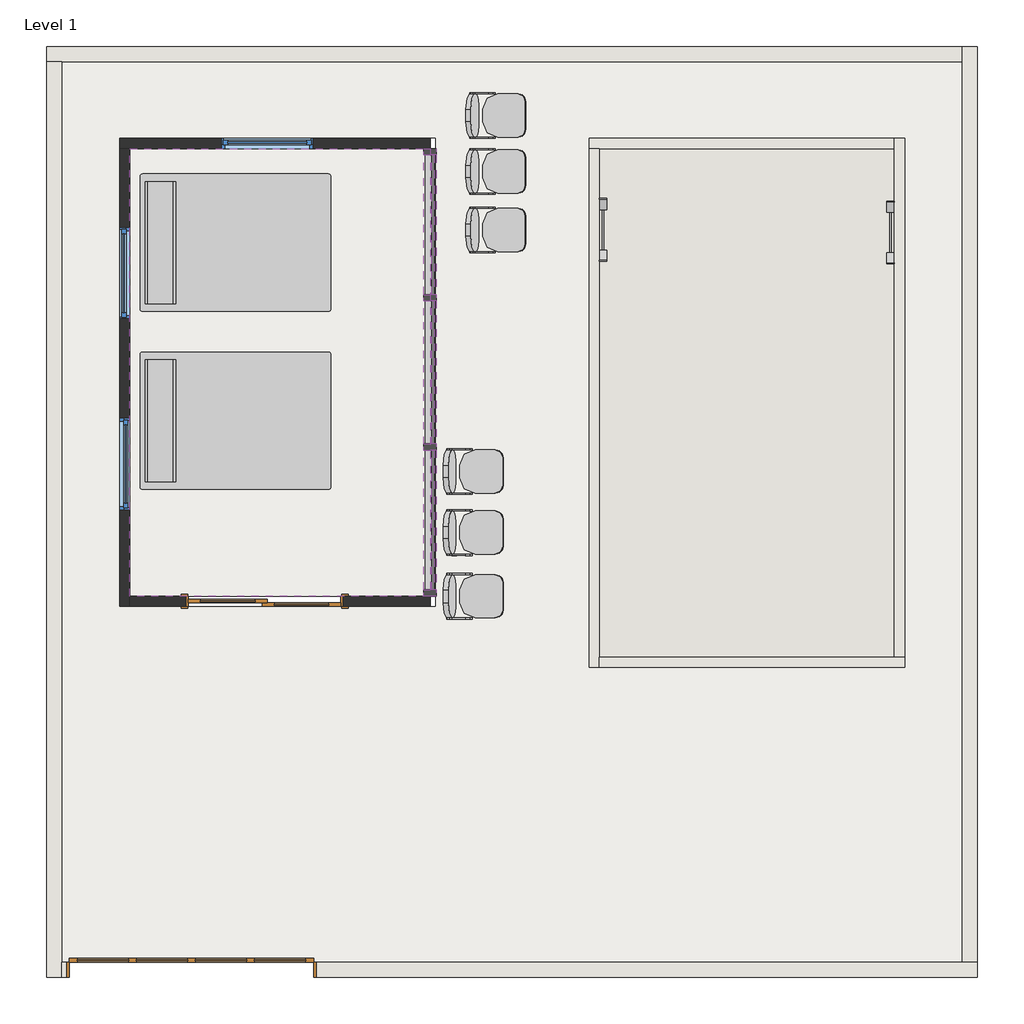
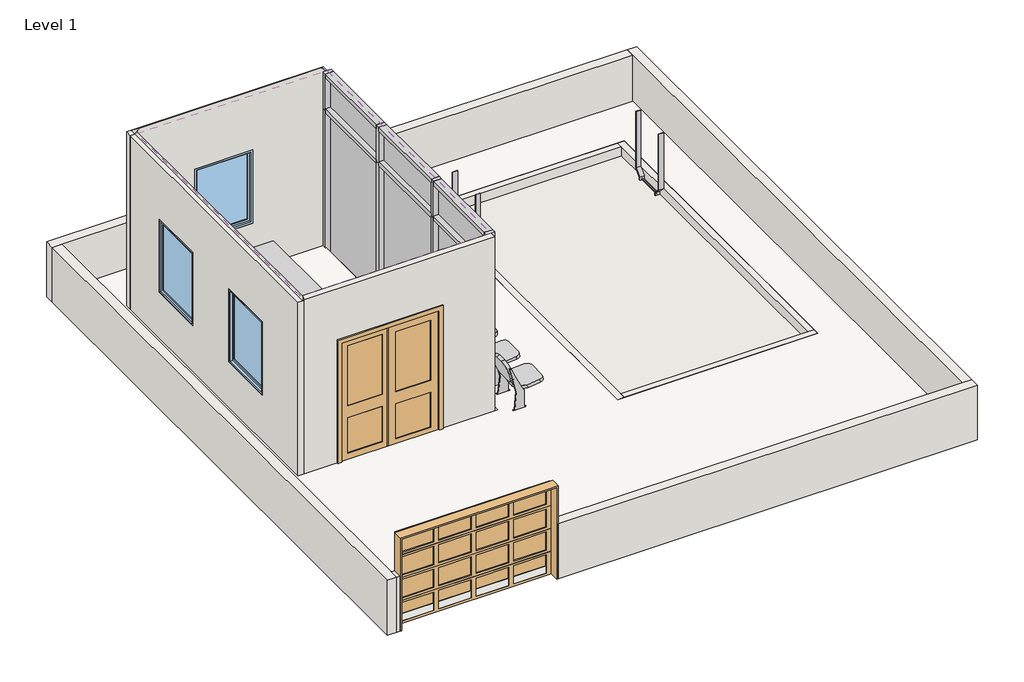
# One storey, incomplete: 17 members, 12 walls, 8 furniture elements, 6 plates, 3 slabs, 3 windows, 2 doors, 2 proxies, 1 covering.
"""IFC4 building model written with IfcOpenShell, lengths in millimetres."""

from ifc_helpers import new_model, si_unit, frame, origin, origin_with_axes, place, context, project, spatial, polyline, outline, extrude, faceted_brep, transform, mapped, element, save
from components import ladder_standard_19ab645e, ladder_standard_86d3c5fc, door_11e1ca51, m_door_interior_double_sliding_2_panel_wood_1524_x_2134mm_74d6d249, furniture_0253826f, m_seating_auditorium_457_x_610mm_3d1d9cbc, member_f0fea5a5, member_6e77e263, member_ee409385, member_47bfaf8a, member_2e151cea, member_16a3b7c2, member_950090be, member_3c30aa5e, system_panel_glazed_1fb160e7, system_panel_glazed_56a6bb10, system_panel_glazed_2f197d06, system_panel_glazed_b12e8a87, walls_1_walls_1_4e806b56, window_d45db805

model = new_model("IFC4")

# Units and contexts
model_context = context("Model", 3, world=origin())
ifc_project = project(units=[si_unit("LENGTHUNIT", "METRE", prefix="MILLI")], contexts=[model_context])

# Site, building, storey
site = spatial("IfcSite", under=ifc_project)
building = spatial("IfcBuilding", under=site)
storey = spatial("IfcBuildingStorey", under=building, Name="Level 1", Elevation=0.0)

# Proxies
placement = place(None, origin())
ladder_standard_shape = ladder_standard_19ab645e(model_context)
element("IfcBuildingElementProxy", 1, Name="Ladder : Standard", ObjectType="Ladder : Standard", at=placement, inside=storey, context=model_context, shape_type="MappedRepresentation", body=[
    mapped(ladder_standard_shape, transform((-3124.1401579, 11504.6599287, 19.05), x_axis=(0.0, 1.0, 0.0), y_axis=(-1.0, 0.0, 0.0), z_axis=(0.0, 0.0, 1.0))),
])
ladder_standard_2_shape = ladder_standard_86d3c5fc(model_context)
element("IfcBuildingElementProxy", 2, Name="Ladder : Standard", ObjectType="Ladder : Standard", at=placement, inside=storey, context=model_context, shape_type="MappedRepresentation", body=[
    mapped(ladder_standard_2_shape, transform((-6197.5401579, 11530.0599287, 0.0), x_axis=(0.0, -1.0, 0.0), y_axis=(1.0, 0.0, 0.0), z_axis=(0.0, 0.0, 1.0))),
])

# Covering
element("IfcCovering", 3, ObjectType="2' x 4' ACT System", at=placement, inside=storey, context=model_context, shape_type="SweptSolid", body=[
    extrude(outline(polyline([(-10822.8289971, 12342.8599287), (-7825.6289971, 12342.8599287), (-7825.6289971, 7872.4599287), (-10822.8289971, 7872.4599287), (-10822.8289971, 12342.8599287)])), frame((0.0, 0.0, 3048.0), z_axis=(0.0, 0.0, 1.0), x_axis=(1.0, 0.0, 0.0)), (0.0, 0.0, 1.0), 57.15),
])

# Doors
door_shape = door_11e1ca51(model_context)
element("IfcDoor", 4, ObjectType="Door-Garage-Embossed_Panel : 96\" x 60\"", at=placement, inside=storey, context=model_context, shape_type="MappedRepresentation", body=[
    mapped(door_shape, transform((-10207.2557492, 4138.1512164, 0.0), x_axis=(-1.0, 0.0, 0.0), y_axis=(0.0, -1.0, 0.0), z_axis=(0.0, 0.0, 1.0))),
])
m_door_interior_double_sliding_2_panel_wood_1524_x_2134mm_shape = m_door_interior_double_sliding_2_panel_wood_1524_x_2134mm_74d6d249(model_context)
element("IfcDoor", 5, ObjectType="M_Door-Interior-Double-Sliding-2_Panel-Wood : 1524 x 2134mm", at=placement, inside=storey, context=model_context, shape_type="MappedRepresentation", body=[
    mapped(m_door_interior_double_sliding_2_panel_wood_1524_x_2134mm_shape, transform((-9476.6289971, 7818.4849287, 0.0), x_axis=(-1.0, 0.0, 0.0), y_axis=(0.0, -1.0, 0.0), z_axis=(0.0, 0.0, 1.0))),
])

# Furniture
furniture_shape = furniture_0253826f(model_context)
element("IfcFurniture", 6, ObjectType="Bed-Standard : Double 54\" x 75\"", at=placement, inside=storey, context=model_context, shape_type="MappedRepresentation", body=[
    mapped(furniture_shape, transform((-9814.324079, 11131.5714041, 152.4), x_axis=(0.0, 1.0000000000000002, 0.0), y_axis=(-1.0000000000000002, 0.0, 0.0), z_axis=(0.0, 0.0, 1.0))),
])
element("IfcFurniture", 7, ObjectType="Bed-Standard : Double 54\" x 75\"", at=placement, inside=storey, context=model_context, shape_type="MappedRepresentation", body=[
    mapped(furniture_shape, transform((-9814.324079, 9353.5714041, 152.4), x_axis=(0.0, 1.0000000000000002, 0.0), y_axis=(-1.0000000000000002, 0.0, 0.0), z_axis=(0.0, 0.0, 1.0))),
])
m_seating_auditorium_457_x_610mm_shape = m_seating_auditorium_457_x_610mm_3d1d9cbc(model_context)
element("IfcFurniture", 8, ObjectType="M_Seating-Auditorium : 457 x 610mm", at=placement, inside=storey, context=model_context, shape_type="MappedRepresentation", body=[
    mapped(m_seating_auditorium_457_x_610mm_shape, transform((-7365.3155677, 12833.7877975, 152.4), x_axis=(0.0, -1.0, 0.0), y_axis=(1.0, 0.0, 0.0), z_axis=(0.0, 0.0, 1.0))),
])
element("IfcFurniture", 9, ObjectType="M_Seating-Auditorium : 457 x 610mm", at=placement, inside=storey, context=model_context, shape_type="MappedRepresentation", body=[
    mapped(m_seating_auditorium_457_x_610mm_shape, transform((-7365.3155677, 12274.9877975, 152.4), x_axis=(0.0, -1.0, 0.0), y_axis=(1.0, 0.0, 0.0), z_axis=(0.0, 0.0, 1.0))),
])
element("IfcFurniture", 10, ObjectType="M_Seating-Auditorium : 457 x 610mm", at=placement, inside=storey, context=model_context, shape_type="MappedRepresentation", body=[
    mapped(m_seating_auditorium_457_x_610mm_shape, transform((-7365.3155677, 11690.7877975, 152.4), x_axis=(0.0, -1.0, 0.0), y_axis=(1.0, 0.0, 0.0), z_axis=(0.0, 0.0, 1.0))),
])
element("IfcFurniture", 11, ObjectType="M_Seating-Auditorium : 457 x 610mm", at=placement, inside=storey, context=model_context, shape_type="MappedRepresentation", body=[
    mapped(m_seating_auditorium_457_x_610mm_shape, transform((-7593.9155677, 9277.7877975, 152.4), x_axis=(0.0, -1.0, 0.0), y_axis=(1.0, 0.0, 0.0), z_axis=(0.0, 0.0, 1.0))),
])
element("IfcFurniture", 12, ObjectType="M_Seating-Auditorium : 457 x 610mm", at=placement, inside=storey, context=model_context, shape_type="MappedRepresentation", body=[
    mapped(m_seating_auditorium_457_x_610mm_shape, transform((-7593.9155677, 8668.1877975, 152.4), x_axis=(0.0, -1.0, 0.0), y_axis=(1.0, 0.0, 0.0), z_axis=(0.0, 0.0, 1.0))),
])
element("IfcFurniture", 13, ObjectType="M_Seating-Auditorium : 457 x 610mm", at=placement, inside=storey, context=model_context, shape_type="MappedRepresentation", body=[
    mapped(m_seating_auditorium_457_x_610mm_shape, transform((-7593.9155677, 8033.1877975, 152.4), x_axis=(0.0, -1.0, 0.0), y_axis=(1.0, 0.0, 0.0), z_axis=(0.0, 0.0, 1.0))),
])

# Members
member_shape = member_f0fea5a5(model_context)
element("IfcMember", 14, ObjectType="Rectangular Mullion : 2.5\" x 5\" rectangular", at=placement, inside=storey, context=model_context, shape_type="MappedRepresentation", body=[
    mapped(member_shape, transform((-7825.6289971, 10852.7265953, 0.0), x_axis=(0.0, -1.0, 0.0), y_axis=(-1.0, 0.0, 0.0), z_axis=(0.0, 0.0, -1.0))),
])
element("IfcMember", 15, ObjectType="Rectangular Mullion : 2.5\" x 5\" rectangular", at=placement, inside=storey, context=model_context, shape_type="MappedRepresentation", body=[
    mapped(member_shape, transform((-7825.6289971, 9362.593262, 0.0), x_axis=(0.0, -1.0, 0.0), y_axis=(-1.0, 0.0, 0.0), z_axis=(0.0, 0.0, -1.0))),
])
member_2_shape = member_6e77e263(model_context)
element("IfcMember", 16, ObjectType="Rectangular Mullion : 2.5\" x 5\" rectangular", at=placement, inside=storey, context=model_context, shape_type="MappedRepresentation", body=[
    mapped(member_2_shape, transform((-7825.6289971, 10852.7265953, 2438.4), x_axis=(0.0, -1.0, 0.0), y_axis=(-1.0, 0.0, 0.0), z_axis=(0.0, 0.0, -1.0))),
])
element("IfcMember", 17, ObjectType="Rectangular Mullion : 2.5\" x 5\" rectangular", at=placement, inside=storey, context=model_context, shape_type="MappedRepresentation", body=[
    mapped(member_2_shape, transform((-7825.6289971, 9362.593262, 2438.4), x_axis=(0.0, -1.0, 0.0), y_axis=(-1.0, 0.0, 0.0), z_axis=(0.0, 0.0, -1.0))),
])
member_3_shape = member_ee409385(model_context)
element("IfcMember", 18, ObjectType="Rectangular Mullion : 2.5\" x 5\" rectangular", at=placement, inside=storey, context=model_context, shape_type="MappedRepresentation", body=[
    mapped(member_3_shape, transform((-7825.6289971, 7872.4599287, 0.0), x_axis=(0.0, -1.0, 0.0), y_axis=(-1.0, 0.0, 0.0), z_axis=(0.0, 0.0, -1.0))),
])
element("IfcMember", 19, ObjectType="Rectangular Mullion : 2.5\" x 5\" rectangular", at=placement, inside=storey, context=model_context, shape_type="MappedRepresentation", body=[
    mapped(member_3_shape, transform((-7825.6289971, 12342.8599287, 2438.4), x_axis=(0.0, 1.0, 0.0), y_axis=(-1.0, 0.0, 0.0), z_axis=(0.0, 0.0, 1.0))),
])
member_4_shape = member_47bfaf8a(model_context)
element("IfcMember", 20, ObjectType="Rectangular Mullion : 2.5\" x 5\" rectangular", at=placement, inside=storey, context=model_context, shape_type="MappedRepresentation", body=[
    mapped(member_4_shape, transform((-7825.6289971, 7872.4599287, 2438.4), x_axis=(0.0, -1.0, 0.0), y_axis=(-1.0, 0.0, 0.0), z_axis=(0.0, 0.0, -1.0))),
])
element("IfcMember", 21, ObjectType="Rectangular Mullion : 2.5\" x 5\" rectangular", at=placement, inside=storey, context=model_context, shape_type="MappedRepresentation", body=[
    mapped(member_4_shape, transform((-7825.6289971, 12342.8599287, 3048.0), x_axis=(0.0, 1.0, 0.0), y_axis=(-1.0, 0.0, 0.0), z_axis=(0.0, 0.0, 1.0))),
])
member_5_shape = member_2e151cea(model_context)
element("IfcMember", 22, ObjectType="Rectangular Mullion : 2.5\" x 5\" rectangular", at=placement, inside=storey, context=model_context, shape_type="MappedRepresentation", body=[
    mapped(member_5_shape, transform((-7825.6289971, 10820.9765953, 0.0), x_axis=(0.0, 0.0, -1.0), y_axis=(-1.0, 0.0, 0.0), z_axis=(0.0, 1.0, 0.0))),
])
member_6_shape = member_16a3b7c2(model_context)
element("IfcMember", 23, ObjectType="Rectangular Mullion : 2.5\" x 5\" rectangular", at=placement, inside=storey, context=model_context, shape_type="MappedRepresentation", body=[
    mapped(member_6_shape, transform((-7825.6289971, 12279.3599287, 0.0), x_axis=(0.0, 0.0, -1.0), y_axis=(-1.0, 0.0, 0.0), z_axis=(0.0, 1.0, 0.0))),
])
element("IfcMember", 24, ObjectType="Rectangular Mullion : 2.5\" x 5\" rectangular", at=placement, inside=storey, context=model_context, shape_type="MappedRepresentation", body=[
    mapped(member_6_shape, transform((-7825.6289971, 9330.843262, 0.0), x_axis=(0.0, 0.0, -1.0), y_axis=(-1.0, 0.0, 0.0), z_axis=(0.0, 1.0, 0.0))),
])
element("IfcMember", 25, ObjectType="Rectangular Mullion : 2.5\" x 5\" rectangular", at=placement, inside=storey, context=model_context, shape_type="MappedRepresentation", body=[
    mapped(member_6_shape, transform((-7825.6289971, 7935.9599287, 3048.0), x_axis=(0.0, 0.0, 1.0), y_axis=(-1.0, 0.0, 0.0), z_axis=(0.0, -1.0, 0.0))),
])
element("IfcMember", 26, ObjectType="Rectangular Mullion : 2.5\" x 5\" rectangular", at=placement, inside=storey, context=model_context, shape_type="MappedRepresentation", body=[
    mapped(member_6_shape, transform((-7825.6289971, 10884.4765953, 3048.0), x_axis=(0.0, 0.0, 1.0), y_axis=(-1.0, 0.0, 0.0), z_axis=(0.0, -1.0, 0.0))),
])
element("IfcMember", 27, ObjectType="Rectangular Mullion : 2.5\" x 5\" rectangular", at=placement, inside=storey, context=model_context, shape_type="MappedRepresentation", body=[
    mapped(member_5_shape, transform((-7825.6289971, 9394.343262, 3048.0), x_axis=(0.0, 0.0, 1.0), y_axis=(-1.0, 0.0, 0.0), z_axis=(0.0, -1.0, 0.0))),
])
member_7_shape = member_950090be(model_context)
element("IfcMember", 28, ObjectType="Rectangular Mullion : 2.5\" x 5\" rectangular", at=placement, inside=storey, context=model_context, shape_type="MappedRepresentation", body=[
    mapped(member_7_shape, transform((-7825.6289971, 10884.4765953, 2438.4), x_axis=(0.0, 0.0, 1.0), y_axis=(-1.0, 0.0, 0.0), z_axis=(0.0, -1.0, 0.0))),
])
element("IfcMember", 29, ObjectType="Rectangular Mullion : 2.5\" x 5\" rectangular", at=placement, inside=storey, context=model_context, shape_type="MappedRepresentation", body=[
    mapped(member_7_shape, transform((-7825.6289971, 7935.9599287, 2438.4), x_axis=(0.0, 0.0, 1.0), y_axis=(-1.0, 0.0, 0.0), z_axis=(0.0, -1.0, 0.0))),
])
member_8_shape = member_3c30aa5e(model_context)
element("IfcMember", 30, ObjectType="Rectangular Mullion : 2.5\" x 5\" rectangular", at=placement, inside=storey, context=model_context, shape_type="MappedRepresentation", body=[
    mapped(member_8_shape, transform((-7825.6289971, 9394.343262, 2438.4), x_axis=(0.0, 0.0, 1.0), y_axis=(-1.0, 0.0, 0.0), z_axis=(0.0, -1.0, 0.0))),
])

# Plates
system_panel_glazed_shape = system_panel_glazed_1fb160e7(model_context)
element("IfcPlate", 31, ObjectType="System Panel : Glazed", at=placement, inside=storey, context=model_context, shape_type="MappedRepresentation", body=[
    mapped(system_panel_glazed_shape, transform((-7825.6289971, 11581.918262, 63.5), x_axis=(0.0, -1.0, 0.0), y_axis=(1.0, 0.0, 0.0), z_axis=(0.0, 0.0, 1.0))),
])
element("IfcPlate", 32, ObjectType="System Panel : Glazed", at=placement, inside=storey, context=model_context, shape_type="MappedRepresentation", body=[
    mapped(system_panel_glazed_shape, transform((-7825.6289971, 8633.4015953, 63.5), x_axis=(0.0, -1.0, 0.0), y_axis=(1.0, 0.0, 0.0), z_axis=(0.0, 0.0, 1.0))),
])
system_panel_glazed_2_shape = system_panel_glazed_56a6bb10(model_context)
element("IfcPlate", 33, ObjectType="System Panel : Glazed", at=placement, inside=storey, context=model_context, shape_type="MappedRepresentation", body=[
    mapped(system_panel_glazed_2_shape, transform((-7825.6289971, 10107.6599287, 63.5), x_axis=(0.0, -1.0, 0.0), y_axis=(1.0, 0.0, 0.0), z_axis=(0.0, 0.0, 1.0))),
])
system_panel_glazed_3_shape = system_panel_glazed_2f197d06(model_context)
element("IfcPlate", 34, ObjectType="System Panel : Glazed", at=placement, inside=storey, context=model_context, shape_type="MappedRepresentation", body=[
    mapped(system_panel_glazed_3_shape, transform((-7825.6289971, 11581.918262, 2470.15), x_axis=(0.0, -1.0, 0.0), y_axis=(1.0, 0.0, 0.0), z_axis=(0.0, 0.0, 1.0))),
])
element("IfcPlate", 35, ObjectType="System Panel : Glazed", at=placement, inside=storey, context=model_context, shape_type="MappedRepresentation", body=[
    mapped(system_panel_glazed_3_shape, transform((-7825.6289971, 8633.4015953, 2470.15), x_axis=(0.0, -1.0, 0.0), y_axis=(1.0, 0.0, 0.0), z_axis=(0.0, 0.0, 1.0))),
])
system_panel_glazed_4_shape = system_panel_glazed_b12e8a87(model_context)
element("IfcPlate", 36, ObjectType="System Panel : Glazed", at=placement, inside=storey, context=model_context, shape_type="MappedRepresentation", body=[
    mapped(system_panel_glazed_4_shape, transform((-7825.6289971, 10107.6599287, 2470.15), x_axis=(0.0, -1.0, 0.0), y_axis=(1.0, 0.0, 0.0), z_axis=(0.0, 0.0, 1.0))),
])

# Slabs
element("IfcSlab", 37, ObjectType="3\"", at=placement, inside=storey, context=model_context, shape_type="SweptSolid", body=[
    extrude(outline(polyline([(-3187.6401579, 12342.8599287), (-3187.6401579, 7262.8599287), (-6134.0401579, 7262.8599287), (-6134.0401579, 12342.8599287), (-3187.6401579, 12342.8599287)])), frame((0.0, 0.0, -1905.0), z_axis=(0.0, 0.0, 1.0), x_axis=(1.0, 0.0, 0.0)), (0.0, 0.0, 1.0), 76.2),
])
element("IfcSlab", 38, ObjectType="4\"", at=placement, inside=storey, context=model_context, shape_type="SweptSolid", body=[
    extrude(outline(polyline([(-7876.4289971, 12342.8599287), (-7876.4289971, 7872.4599287), (-10822.8289971, 7872.4599287), (-10822.8289971, 12342.8599287), (-7876.4289971, 12342.8599287)])), frame((0.0, 0.0, 50.8), z_axis=(0.0, 0.0, 1.0), x_axis=(1.0, 0.0, 0.0)), (0.0, 0.0, 1.0), 101.6),
])
element("IfcSlab", 39, ObjectType="6\"", at=placement, inside=storey, context=model_context, shape_type="SweptSolid", body=[
    extrude(outline(polyline([(-11502.6557492, 13209.1262164), (-2511.0557492, 13209.1262164), (-2511.0557492, 4217.5262164), (-11502.6557492, 4217.5262164), (-11502.6557492, 13209.1262164)]), holes=[polyline([(-3086.0401579, 7161.2599287), (-3086.0401579, 12444.4599287), (-6235.6401579, 12444.4599287), (-6235.6401579, 7161.2599287), (-3086.0401579, 7161.2599287)]), polyline([(-7774.8289971, 12444.4599287), (-10924.4289971, 12444.4599287), (-10924.4289971, 7770.8599287), (-7774.8289971, 7770.8599287), (-7774.8289971, 12444.4599287)])]), origin_with_axes(), (0.0, 0.0, 1.0), 152.4),
])

# Walls
element("IfcWall", 40, ObjectType="4\"", at=placement, inside=storey, context=model_context, shape_type="Brep", body=[
    faceted_brep([(-10924.4289971, 12342.8599287, 0.0), (-10822.8289971, 12342.8599287, 0.0), (-7825.6289971, 12342.8599287, 0.0), (-7825.6289971, 12342.8599287, 3048.0), (-7848.8563022, 12342.8599287, 3048.0), (-7914.5243913, 12342.8599287, 3124.2), (-10784.7336028, 12342.8599287, 3124.2), (-10822.8289971, 12342.8599287, 3079.99483), (-10850.401692, 12342.8599287, 3048.0), (-10924.4289971, 12342.8599287, 3048.0), (-8994.0289971, 12342.8599287, 2133.6), (-8994.0289971, 12342.8599287, 914.4), (-9908.4289971, 12342.8599287, 914.4), (-9908.4289971, 12342.8599287, 2133.6), (-10924.4289971, 12444.4599287, 0.0), (-10924.4289971, 12444.4599287, 3048.0), (-10850.401692, 12444.4599287, 3048.0), (-7848.8563022, 12444.4599287, 3048.0), (-7825.6289971, 12444.4599287, 3048.0), (-7825.6289971, 12444.4599287, 0.0), (-8994.0289971, 12444.4599287, 2133.6), (-9908.4289971, 12444.4599287, 2133.6), (-9908.4289971, 12444.4599287, 914.4), (-8994.0289971, 12444.4599287, 914.4)], [[[0, 1, 2, 3, 4, 5, 6, 7, 8, 9], [10, 11, 12, 13]], [[14, 15, 16, 17, 18, 19], [20, 21, 22, 23]], [[2, 1, 0, 14, 19]], [[3, 2, 19, 18]], [[0, 9, 15, 14]], [[9, 8, 16, 15]], [[8, 7, 6, 16]], [[6, 5, 17, 16]], [[5, 4, 17]], [[4, 3, 18, 17]], [[11, 10, 20, 23]], [[12, 11, 23, 22]], [[13, 12, 22, 21]], [[10, 13, 21, 20]]]),
])
element("IfcWall", 41, ObjectType="4\"", at=placement, inside=storey, context=model_context, shape_type="Brep", body=[
    faceted_brep([(-10822.8289971, 7770.8599287, 0.0), (-10822.8289971, 7872.4599287, 0.0), (-10822.8289971, 12342.8599287, 0.0), (-10822.8289971, 12342.8599287, 3079.99483), (-10822.8289971, 7813.5197021, 3079.99483), (-10822.8289971, 7770.8599287, 3048.0), (-10822.8289971, 8736.0599287, 2133.6), (-10822.8289971, 9650.4599287, 2133.6), (-10822.8289971, 9650.4599287, 914.4), (-10822.8289971, 8736.0599287, 914.4), (-10822.8289971, 11555.4599287, 2133.6), (-10822.8289971, 11555.4599287, 914.4), (-10822.8289971, 10641.0599287, 914.4), (-10822.8289971, 10641.0599287, 2133.6), (-10924.4289971, 7770.8599287, 0.0), (-10924.4289971, 7770.8599287, 3048.0), (-10924.4289971, 12342.8599287, 3048.0), (-10924.4289971, 12342.8599287, 0.0), (-10924.4289971, 8736.0599287, 2133.6), (-10924.4289971, 8736.0599287, 914.4), (-10924.4289971, 9650.4599287, 914.4), (-10924.4289971, 9650.4599287, 2133.6), (-10924.4289971, 11555.4599287, 2133.6), (-10924.4289971, 10641.0599287, 2133.6), (-10924.4289971, 10641.0599287, 914.4), (-10924.4289971, 11555.4599287, 914.4), (-10850.401692, 12342.8599287, 3048.0), (-10850.401692, 7770.8599287, 3048.0)], [[[0, 1, 2, 3, 4, 5], [6, 7, 8, 9], [10, 11, 12, 13]], [[14, 15, 16, 17], [18, 19, 20, 21], [22, 23, 24, 25]], [[2, 1, 0, 14, 17]], [[3, 2, 17, 16, 26]], [[5, 4, 27]], [[4, 3, 26, 27]], [[26, 16, 15, 27]], [[0, 5, 27, 15, 14]], [[19, 18, 6, 9]], [[20, 19, 9, 8]], [[21, 20, 8, 7]], [[18, 21, 7, 6]], [[11, 10, 22, 25]], [[12, 11, 25, 24]], [[13, 12, 24, 23]], [[10, 13, 23, 22]]]),
])
element("IfcWall", 42, ObjectType="4\"", at=placement, inside=storey, context=model_context, shape_type="SweptSolid", body=[
    extrude(outline(polyline([(0.0, -7825.6289971), (3048.0, -7825.6289971), (3048.0, -10822.8289971), (0.0, -10822.8289971), (0.0, -10263.6289971), (2158.6, -10263.6289971), (2158.6, -8689.6289971), (0.0, -8689.6289971), (0.0, -7825.6289971)])), frame((0.0, 7770.8599287, 0.0), z_axis=(0.0, 1.0, 0.0), x_axis=(0.0, 0.0, 1.0)), (0.0, 0.0, 1.0), 101.6),
])
element("IfcWall", 43, ObjectType="4\" 2", at=placement, inside=storey, context=model_context, shape_type="Brep", body=[
    faceted_brep([(-6235.6401579, 12342.8599287, -1828.8), (-6134.0401579, 12342.8599287, -1828.8), (-3187.6401579, 12342.8599287, -1828.8), (-3187.6401579, 12342.8599287, 152.4), (-6134.0401579, 12342.8599287, 152.4), (-6235.6401579, 12342.8599287, 152.4), (-6235.6401579, 12444.4599287, -1828.8), (-6235.6401579, 12444.4599287, 152.4), (-3187.6401579, 12444.4599287, 152.4), (-3187.6401579, 12444.4599287, -1828.8)], [[[0, 1, 2, 3, 4, 5]], [[6, 7, 8, 9]], [[2, 1, 0, 6, 9]], [[5, 4, 3, 8, 7]], [[0, 5, 7, 6]], [[3, 2, 9, 8]]]),
])
element("IfcWall", 44, ObjectType="4\" 2", at=placement, inside=storey, context=model_context, shape_type="Brep", body=[
    faceted_brep([(-6134.0401579, 7161.2599287, -1828.8), (-6134.0401579, 7262.8599287, -1828.8), (-6134.0401579, 12342.8599287, -1828.8), (-6134.0401579, 12342.8599287, 152.4), (-6134.0401579, 7262.8599287, 152.4), (-6134.0401579, 7161.2599287, 152.4), (-6235.6401579, 7161.2599287, -1828.8), (-6235.6401579, 7161.2599287, 152.4), (-6235.6401579, 12342.8599287, 152.4), (-6235.6401579, 12342.8599287, -1828.8)], [[[0, 1, 2, 3, 4, 5]], [[6, 7, 8, 9]], [[2, 1, 0, 6, 9]], [[5, 4, 3, 8, 7]], [[0, 5, 7, 6]], [[3, 2, 9, 8]]]),
])
element("IfcWall", 45, ObjectType="4\" 2", at=placement, inside=storey, context=model_context, shape_type="Brep", body=[
    faceted_brep([(-3086.0401579, 7262.8599287, -1828.8), (-3187.6401579, 7262.8599287, -1828.8), (-6134.0401579, 7262.8599287, -1828.8), (-6134.0401579, 7262.8599287, 152.4), (-3187.6401579, 7262.8599287, 152.4), (-3086.0401579, 7262.8599287, 152.4), (-3086.0401579, 7161.2599287, -1828.8), (-3086.0401579, 7161.2599287, 152.4), (-6134.0401579, 7161.2599287, 152.4), (-6134.0401579, 7161.2599287, -1828.8)], [[[0, 1, 2, 3, 4, 5]], [[6, 7, 8, 9]], [[2, 1, 0, 6, 9]], [[5, 4, 3, 8, 7]], [[0, 5, 7, 6]], [[3, 2, 9, 8]]]),
])
element("IfcWall", 46, ObjectType="4\" 2", at=placement, inside=storey, context=model_context, shape_type="Brep", body=[
    faceted_brep([(-3187.6401579, 12444.4599287, -1828.8), (-3187.6401579, 12342.8599287, -1828.8), (-3187.6401579, 7262.8599287, -1828.8), (-3187.6401579, 7262.8599287, 152.4), (-3187.6401579, 12342.8599287, 152.4), (-3187.6401579, 12444.4599287, 152.4), (-3086.0401579, 12444.4599287, -1828.8), (-3086.0401579, 12444.4599287, 152.4), (-3086.0401579, 7262.8599287, 152.4), (-3086.0401579, 7262.8599287, -1828.8)], [[[0, 1, 2, 3, 4, 5]], [[6, 7, 8, 9]], [[2, 1, 0, 6, 9]], [[5, 4, 3, 8, 7]], [[0, 5, 7, 6]], [[3, 2, 9, 8]]]),
])
element("IfcWall", 47, ObjectType="6\"", at=placement, inside=storey, context=model_context, shape_type="Brep", body=[
    faceted_brep([(-11655.0557492, 13209.1262164, 0.0), (-11502.6557492, 13209.1262164, 0.0), (-2511.0557492, 13209.1262164, 0.0), (-2511.0557492, 13209.1262164, 914.4), (-11502.6557492, 13209.1262164, 914.4), (-11655.0557492, 13209.1262164, 914.4), (-11655.0557492, 13361.5262164, 0.0), (-11655.0557492, 13361.5262164, 914.4), (-2511.0557492, 13361.5262164, 914.4), (-2511.0557492, 13361.5262164, 0.0)], [[[0, 1, 2, 3, 4, 5]], [[6, 7, 8, 9]], [[2, 1, 0, 6, 9]], [[5, 4, 3, 8, 7]], [[0, 5, 7, 6]], [[3, 2, 9, 8]]]),
])
element("IfcWall", 48, ObjectType="6\"", at=placement, inside=storey, context=model_context, shape_type="Brep", body=[
    faceted_brep([(-11502.6557492, 4065.1262164, 0.0), (-11502.6557492, 4217.5262164, 0.0), (-11502.6557492, 13209.1262164, 0.0), (-11502.6557492, 13209.1262164, 914.4), (-11502.6557492, 4217.5262164, 914.4), (-11502.6557492, 4065.1262164, 914.4), (-11655.0557492, 4065.1262164, 0.0), (-11655.0557492, 4065.1262164, 914.4), (-11655.0557492, 13209.1262164, 914.4), (-11655.0557492, 13209.1262164, 0.0)], [[[0, 1, 2, 3, 4, 5]], [[6, 7, 8, 9]], [[2, 1, 0, 6, 9]], [[5, 4, 3, 8, 7]], [[0, 5, 7, 6]], [[3, 2, 9, 8]]]),
])
element("IfcWall", 49, ObjectType="6\"", at=placement, inside=storey, context=model_context, shape_type="Brep", body=[
    faceted_brep([(-11502.6557492, 4217.5262164, 0.0), (-11502.6557492, 4217.5262164, 914.4), (-11451.8557492, 4217.5262164, 914.4), (-11451.8557492, 4217.5262164, 0.0), (-11502.6557492, 4065.1262164, 914.4), (-11502.6557492, 4065.1262164, 0.0), (-11451.8557492, 4065.1262164, 0.0), (-11451.8557492, 4065.1262164, 914.4)], [[[0, 1, 2, 3]], [[4, 5, 6, 7]], [[5, 0, 3, 6]], [[1, 4, 7, 2]], [[1, 0, 5, 4]], [[3, 2, 7, 6]]]),
    faceted_brep([(-2358.6557492, 4217.5262164, 914.4), (-2358.6557492, 4217.5262164, 0.0), (-2511.0557492, 4217.5262164, 0.0), (-8962.6557492, 4217.5262164, 0.0), (-8962.6557492, 4217.5262164, 914.4), (-2511.0557492, 4217.5262164, 914.4), (-2358.6557492, 4065.1262164, 0.0), (-2358.6557492, 4065.1262164, 914.4), (-8962.6557492, 4065.1262164, 914.4), (-8962.6557492, 4065.1262164, 0.0)], [[[0, 1, 2, 3, 4, 5]], [[6, 7, 8, 9]], [[1, 6, 9, 3, 2]], [[7, 0, 5, 4, 8]], [[1, 0, 7, 6]], [[4, 3, 9, 8]]]),
])
element("IfcWall", 50, ObjectType="6\"", at=placement, inside=storey, context=model_context, shape_type="Brep", body=[
    faceted_brep([(-2511.0557492, 13361.5262164, 0.0), (-2511.0557492, 13209.1262164, 0.0), (-2511.0557492, 4217.5262164, 0.0), (-2511.0557492, 4217.5262164, 914.4), (-2511.0557492, 13209.1262164, 914.4), (-2511.0557492, 13361.5262164, 914.4), (-2358.6557492, 13361.5262164, 0.0), (-2358.6557492, 13361.5262164, 914.4), (-2358.6557492, 4217.5262164, 914.4), (-2358.6557492, 4217.5262164, 0.0)], [[[0, 1, 2, 3, 4, 5]], [[6, 7, 8, 9]], [[2, 1, 0, 6, 9]], [[5, 4, 3, 8, 7]], [[0, 5, 7, 6]], [[3, 2, 9, 8]]]),
])
walls_1_walls_1_shape = walls_1_walls_1_4e806b56(model_context)
element("IfcWall", 51, ObjectType="Walls 1 : Walls 1", at=placement, inside=storey, context=model_context, shape_type="MappedRepresentation", body=[
    mapped(walls_1_walls_1_shape, transform((0.0, 0.0, 0.0), x_axis=(1.0, 0.0, 0.0), y_axis=(0.0, 1.0, 0.0), z_axis=(0.0, 0.0, 1.0))),
])

# Windows
window_shape = window_d45db805(model_context)
element("IfcWindow", 52, ObjectType="Fixed : 36\" x 48\"", at=placement, inside=storey, context=model_context, shape_type="MappedRepresentation", body=[
    mapped(window_shape, transform((-10873.6289971, 9155.1599287, 0.0), x_axis=(0.0, -1.0, 0.0), y_axis=(1.0, 0.0, 0.0), z_axis=(0.0, 0.0, 1.0))),
])
element("IfcWindow", 53, ObjectType="Fixed : 36\" x 48\"", at=placement, inside=storey, context=model_context, shape_type="MappedRepresentation", body=[
    mapped(window_shape, transform((-10873.6289971, 11136.3599287, 0.0), x_axis=(0.0, 1.0, 0.0), y_axis=(-1.0, 0.0, 0.0), z_axis=(0.0, 0.0, 1.0))),
])
element("IfcWindow", 54, ObjectType="Fixed : 36\" x 48\"", at=placement, inside=storey, context=model_context, shape_type="MappedRepresentation", body=[
    mapped(window_shape, transform((-9413.1289971, 12393.6599287, 0.0), x_axis=(1.0, 0.0, 0.0), y_axis=(0.0, 1.0, 0.0), z_axis=(0.0, 0.0, 1.0))),
])

save(model, "model.ifc")

# Revit data of these elements
# Type "Ladder : Standard"
#   Rung Radius = 0' - 0 3/8"
#   Rung Length [instance default] = 1' - 4"
#   Side Rail Thickness = 0' - 3"
#   Side Rail Width = 0' - 0 3/8"
#   Half Guardrail Height = 1' - 9"
#   Height [instance default] = 15' - 2 1/2"
#   Guardrail Length = 1' - 8"
#   Guardrail Height = 3' - 6"
#   Distance [instance default] = 0' - 7"
#   Rung Space [instance default] = 1' - 0"
#   Number of Rungs [instance default] = 15
#   Default Elevation = 0
# Type "2' x 4' ACT System"
#   Assembly Code = "C3030210"
#   built-in parameter 1002203 = 1 (stored number, unit not read)
#   built-in parameter 1002202 = 1 (stored number, unit not read)
#   Layers, outside or top first: 0' - 1 5/8" "Default" (function 1); 0' - 0 5/8" "INT WALL" (function 5)
# Type "Door-Garage-Embossed_Panel : 96\" x 60\""
#   Type Mark = "10"
#   Assembly Code = "B2030400"
#   Analytic Construction = "Metal"
#   Thickness = 0' - 1 1/2"
#   Thermal Resistance (R) = 1.5338 (h·ft²·°F)/BTU
#   Rough Width = 8' - 2"
#   Rough Height = 5' - 1"
#   Panel Height = 1' - 3"
#   Height = 5' - 0"
#   Width = 8' - 0"
#   Heat Transfer Coefficient (U) = 0.6520 BTU/(h·ft²·°F)
#   Panels = 4
#   Function = 1
#   Exterior Trim [instance default] = yes
#   Trim Material = Steel, Paint Finish, Ivory, Matte
#   Panel Material = Steel, Paint Finish, Ivory, Matte
#   Frame Material = Steel, Paint Finish, Ivory, Matte
#   Visual Light Transmittance = 0
#   Solar Heat Gain Coefficient = 0
#   Wall Closure = (empty or 0)
# Type "M_Door-Interior-Double-Sliding-2_Panel-Wood : 1524 x 2134mm"
#   Type Mark = "9"
#   Assembly Code = "C1020300"
#   Analytic Construction = "Wooden"
#   Top Rail = 0' - 4.72441"
#   Thickness = 0' - 1.37795"
#   Thermal Resistance (R) = 2.5876 (h·ft²·°F)/BTU
#   Stiles = 0' - 4.72441"
#   Rough Width = 5' - 1.9685"
#   Rough Height = 7' - 0.98425"
#   Lock Rail = 0' - 7.87402"
#   Height = 7' - 0"
#   Width = 5' - 0"
#   Heat Transfer Coefficient (U) = 0.3865 BTU/(h·ft²·°F)
#   Bottom Rail = 0' - 9.05512"
#   Trim Material = Cherry
#   Panel Material = Cherry
#   Frame Material = Cherry
#   Visual Light Transmittance = 0
#   Solar Heat Gain Coefficient = 0
#   Wall Closure = (empty or 0)
#   Function = (empty or 0)
# Type "Bed-Standard : Double 54\" x 75\""
#   Assembly Code = "E2020200"
#   Length = 6' - 3"
#   Width = 4' - 6"
#   Leg Material = Steel, Chrome Plated
#   Mattress Material = Linen, White
#   Default Elevation = 0
# Type "M_Seating-Auditorium : 457 x 610mm"
#   Seat/Back Material = Linen, Beige
#   Frame Material = Steel, Paint Finish, Dark Gray, Matte
#   Default Elevation = 0
# Type "Rectangular Mullion : 2.5\" x 5\" rectangular"
#   built-in parameter 1007304 = 0.416667 (stored number, unit not read)
#   built-in parameter 1007301 = 0.104167 (stored number, unit not read)
#   built-in parameter 1007300 = 0.104167 (stored number, unit not read)
# Type "System Panel : Glazed"
#   Construction Type Id = "GSP4R"
#   Analytic Construction = "1/8 in Pilkington single glazing"
#   Visual Light Transmittance = 0.9
#   Solar Heat Gain Coefficient = 0.86
#   Heat Transfer Coefficient (U) = 1.18115 BTU/(h·ft²·°F)
# Type "3\""
#   Assembly Code = "B1010"
#   Function = 0
#   Layers, outside or top first: 0' - 3" "TILES" (function 1)
# Type "4\""
#   Assembly Code = "B1010"
#   Function = 0
#   Layers, outside or top first: 0' - 4" "Softwood, Lumber" (function 1)
# Type "6\""
#   Assembly Code = "B1010"
#   Function = 0
#   Layers, outside or top first: 0' - 6" "grass" (function 1)
# Type "4\""
#   Assembly Code = "B2010"
#   Layers, outside or top first: 0' - 4" "INT WALL" (function 1)
# Type "4\" 2"
#   Assembly Code = "B2010"
#   Layers, outside or top first: 0' - 4" "TILES" (function 1)
# Type "6\""
#   Assembly Code = "B2010"
#   Layers, outside or top first: 0' - 6" no material (function 1)
# Type "Fixed : 36\" x 48\""
#   Type Mark = "1"
#   Construction Type Id = "GSP4R"
#   Assembly Code = "B2020100"
#   Analytic Construction = "1/8 in Pilkington single glazing"
#   Visual Light Transmittance = 0.9
#   Solar Heat Gain Coefficient = 0.78
#   Heat Transfer Coefficient (U) = 0.6496 BTU/(h·ft²·°F)
#   Height = 4' - 0"
#   Default Sill Height = 3' - 0"
#   Width = 3' - 0"
#   Window Inset = 0' - 0 3/4"
#   Define Thermal Properties by = 1
#   Glass Pane Material = Glass
#   Sash Material = Sash
#   Wall Closure = (empty or 0)
# Element 1 (IfcBuildingElementProxy, "Ladder : Standard")
#   Rung Space = 1' - 0"
#   Rung Length = 1' - 4"
#   Height = 6' - 0"
#   Distance = 0' - 1.54208"
#   Number of Rungs = 6
#   Phase Created = New Construction
# Element 2 (IfcBuildingElementProxy, "Ladder : Standard")
#   Rung Space = 1' - 0"
#   Rung Length = 1' - 4"
#   Height = 6' - 0"
#   Distance = 0' - 1 25/64"
#   Number of Rungs = 6
#   Phase Created = New Construction
# Element 3 (IfcCovering, "2' x 4' ACT System")
#   Height Offset From Level = 10' - 0"
#   Phase Created = New Construction
#   Materials on its faces: "INT WALL", "Default"
# Element 4 (IfcDoor, "Door-Garage-Embossed_Panel : 96\" x 60\"")
#   Exterior Trim = yes
#   Phase Created = New Construction
#   Materials on its faces: "Steel, Paint Finish, Ivory, Matte"
# Element 5 (IfcDoor, "M_Door-Interior-Double-Sliding-2_Panel-Wood : 1524 x 2134mm")
#   Phase Created = New Construction
#   Materials on its faces: "Cherry"
# Elements 6, 7 (IfcFurniture, "Bed-Standard : Double 54\" x 75\"")
#   Phase Created = New Construction
#   Materials on its faces: "Linen, White", "Steel, Chrome Plated"
# Elements 8, 9, 10, 11, 12, 13 (IfcFurniture, "M_Seating-Auditorium : 457 x 610mm")
#   Phase Created = New Construction
#   Materials on its faces: "Steel, Paint Finish, Dark Gray, Matte", "Linen, Beige"
# Elements 14, 15, 16, 17, 18, 19, 20, 21, 22, 23, 24, 25, 26, 27, 28, 29, 30 (IfcMember, "Rectangular Mullion : 2.5\" x 5\" rectangular")
#   Phase Created = New Construction
#   Materials on its faces: "Aluminum"
# Elements 31, 32, 33, 34, 35, 36 (IfcPlate, "System Panel : Glazed")
#   Phase Created = New Construction
#   Materials on its faces: "Glass"
# Element 37 (IfcSlab, "3\"")
#   Height Offset From Level = -6' - 0"
#   Phase Created = New Construction
#   Materials on its faces: "TILES"
# Element 38 (IfcSlab, "4\"")
#   Height Offset From Level = 0' - 6"
#   Phase Created = New Construction
#   Materials on its faces: "Softwood, Lumber"
# Element 39 (IfcSlab, "6\"")
#   built-in parameter 1001955 = 1.5708 (stored number, unit not read)
#   Height Offset From Level = 0' - 6"
#   Phase Created = New Construction
#   Materials on its faces: "grass"
# Elements 40, 41, 42 (IfcWall, "4\"")
#   Top Offset = 0' - 0"
#   Base Offset = 0' - 0"
#   Unconnected Height = 10' - 0"
#   wall height = 10' - 0"
#   Phase Created = New Construction
#   Base Constraint = Level 1
#   Materials on its faces: "INT WALL"
# Elements 43, 44, 45, 46 (IfcWall, "4\" 2")
#   built-in parameter 1001111 = -6' - 0"
#   Top Offset = 0' - 0"
#   Base Offset = -6' - 0"
#   Unconnected Height = 6' - 6"
#   wall height = 6' - 6"
#   Phase Created = New Construction
#   Base Constraint = Level 1
#   Materials on its faces: "TILES"
# Elements 47, 48, 49, 50 (IfcWall, "6\"")
#   Top Offset = 0' - 0"
#   Base Offset = 0' - 0"
#   Unconnected Height = 3' - 0"
#   wall height = 3' - 0"
#   Phase Created = New Construction
#   Base Constraint = Level 1
#   Materials on its faces: "Default Wall"
# Element 51 (IfcWall, "Walls 1 : Walls 1")
#   Phase Created = New Construction
#   Materials on its faces: "WATER"
# Element 52 (IfcWindow, "Fixed : 36\" x 48\"")
#   Mark = "1"
#   Phase Created = New Construction
#   Materials on its faces: "Sash", "Glass"
# Element 53 (IfcWindow, "Fixed : 36\" x 48\"")
#   Mark = "2"
#   Phase Created = New Construction
#   Materials on its faces: "Sash", "Glass"
# Element 54 (IfcWindow, "Fixed : 36\" x 48\"")
#   Mark = "3"
#   Phase Created = New Construction
#   Materials on its faces: "Sash", "Glass"
# Materials
#   "Default": colour RGB 127 127 127, transparency 0
#   "INT WALL": class "Generic", colour RGB 148 123 98, transparency 0, Cost = 0
#   "Steel, Paint Finish, Ivory, Matte": class "Metal", colour RGB 247 247 239, transparency 0, Description = "Steel, paint finish, ivory, matte", Cost = 0
#   "Cherry": class "Wood", colour RGB 226 177 128, transparency 0, Description = "Prunus Serotina", Cost = 0
#   "Steel, Chrome Plated": class "Metal", colour RGB 17 17 17, transparency 0, Description = "Chromiuim plated steel", Cost = 0
#   "Linen, White": class "Textile", colour RGB 247 247 239, transparency 0, Description = "Linen, white", Cost = 0
#   "Linen, Beige": class "Textile", colour RGB 249 239 230, transparency 0, Description = "Linen, beige", Cost = 0
#   "Steel, Paint Finish, Dark Gray, Matte": class "Metal", colour RGB 0 0 0, transparency 0, Description = "Steel, paint finish, dark gray, matte", Cost = 0
#   "TILES": class "Generic", colour RGB 99 118 138, transparency 0, Cost = 0
#   "Softwood, Lumber": class "Wood", colour RGB 223 192 134, transparency 0, Description = "Pinus Echinata", Cost = 0
#   "grass": class "Generic", colour RGB 127 136 91, transparency 0, Cost = 0
#   "Glass": class "Glass", colour RGB 0 128 192, transparency 0.75, Description = "Soda Lime Glass", Cost = 0
#   "Sash": class "Wood", colour RGB 224 178 126, transparency 0
#   "Aluminum": class "Metal", colour RGB 247 247 247, transparency 0, Description = "Aluminum 6061", Cost = 0
#   "Default Wall": colour RGB 128 128 128, transparency 0
#   "WATER": class "Generic", colour RGB 0 4 10, transparency 0.08, Cost = 0
